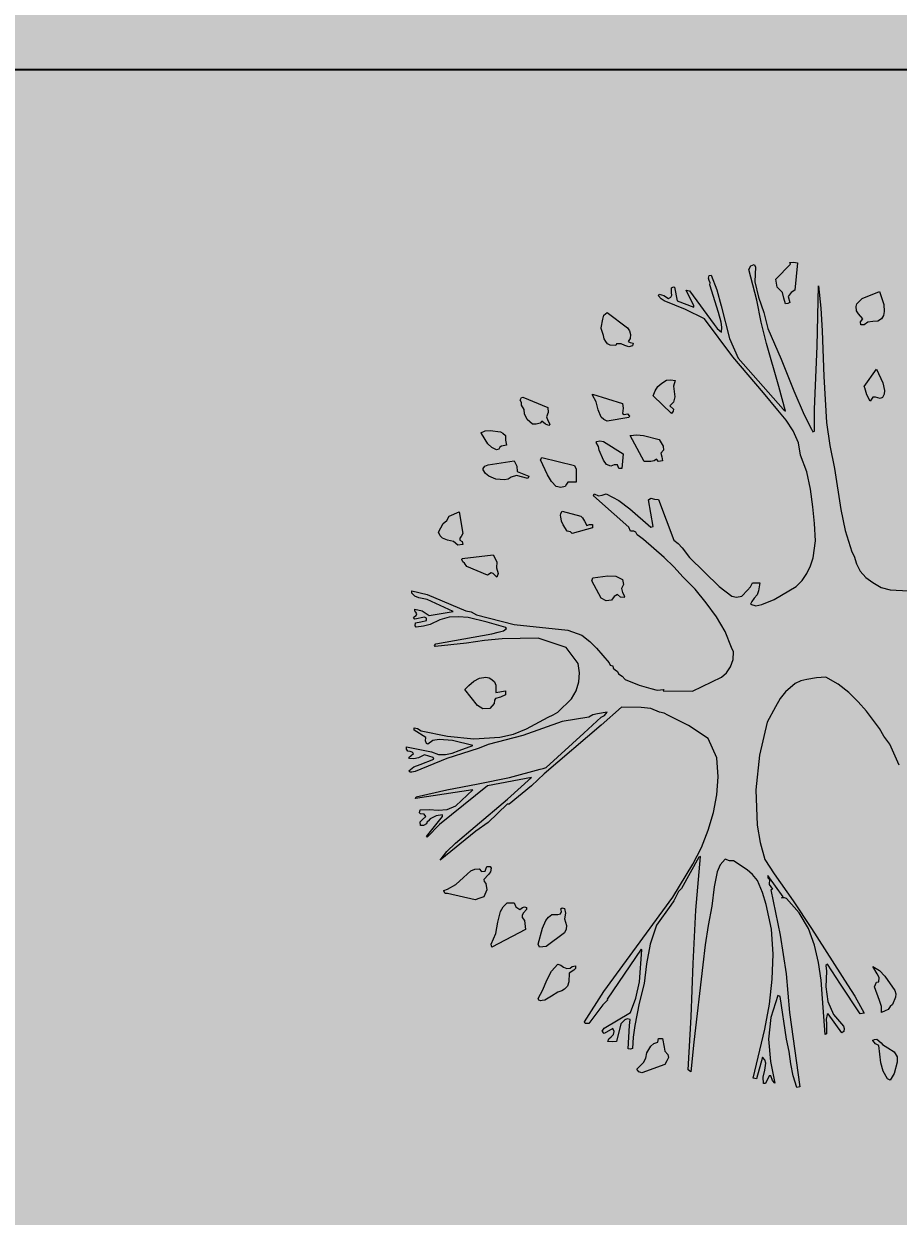
# Model space of a CAD drawing. Units: inches. Extents: x 84 to 1044, y -280 to 906.
# Tile 95 of 105: x 779 to 804, y 479 to 512. Entities that reach past the tile are written whole.
import ezdxf

# ---------------------------------------------------------------- set-up
doc = ezdxf.new("R2010")
doc.units = ezdxf.units.IN
for name, color, linetype, lineweight in [('A-ANNO-DIMS', 2, 'Continuous', 18), ('L-PLNT', 114, 'Continuous', 15), ('WALL', 250, 'Continuous', 35)]:
    doc.layers.add(name, color=color, linetype=linetype, lineweight=lineweight)
doc.layers.add('A-WALL-PATT', color=251, linetype='Continuous', lineweight=9, true_color=0x636466)
doc.layers.add('L-PLNT-PATT', color=9, linetype='Continuous', lineweight=9, true_color=0xafd9aa)
doc.styles.get("Standard").update_dxf_attribs({"font": 'arial.ttf'})
doc.dimstyles.get("Standard").update_dxf_attribs({"dimtxt": 0.18, "dimasz": 0.18, "dimexe": 0.18, "dimexo": 0.0625, "dimgap": 0.09, "dimtad": 0, "dimtih": 1, "dimtoh": 1, "dimdec": 4, "dimzin": 0, "dimdsep": 46, "dimtxsty": 'Standard', "dimcen": 0.09, "dimadec": 0, "dimazin": 0, "dimtfac": 1, "dimtdec": 4, "dimtofl": 0, "dimtmove": 0, "dimatfit": 3, "dimfxl": 1, "dimtolj": 1, "dimtzin": 0, "dimarcsym": 0})

# ---------------------------------------------------------------- blocks, each defined once
blk = doc.blocks.new('A$C37E508DF')
for p, q in [((0.6367, 1.5175), (0.6423, 1.5201)), ((0.6423, 1.5201), (0.6453, 1.5158)), ((0.6826, 1.493), (0.7096, 1.5209)), ((0.7083, 1.5239), (0.7152, 1.5244)), ((0.7096, 1.5209), (0.7083, 1.5239)), ((0.7152, 1.5244), (0.7225, 1.5231)), ((0.7225, 1.5231), (0.7174, 1.4729)), ((0.5583, 1.4948), (0.5596, 1.4995)), ((0.5596, 1.4995), (0.563, 1.5003)), ((0.563, 1.5003), (0.5737, 1.4733)), ((0.6329, 1.5111), (0.6367, 1.5175)), ((0.6475, 1.4545), (0.6329, 1.5111)), ((0.6453, 1.5158), (0.644, 1.4879)), ((0.4897, 1.4772), (0.4935, 1.4789)), ((0.4897, 1.4678), (0.4897, 1.4772)), ((0.4935, 1.4789), (0.4952, 1.478)), ((0.4952, 1.478), (0.5004, 1.4532)), ((0.5596, 1.4905), (0.5583, 1.4948)), ((0.5613, 1.4862), (0.5596, 1.4905)), ((0.5608, 1.4823), (0.5613, 1.4862)), ((0.5767, 1.4317), (0.5608, 1.4823)), ((0.644, 1.4879), (0.6505, 1.46)), ((0.6852, 1.4785), (0.6826, 1.493)), ((0.6946, 1.4682), (0.6852, 1.4785)), ((0.7589, 1.3691), (0.7615, 1.481)), ((0.7615, 1.481), (0.7658, 1.4395)), ((0.4657, 1.4622), (0.4669, 1.4652)), ((0.4708, 1.4566), (0.4657, 1.4622)), ((0.4669, 1.4652), (0.4755, 1.463)), ((0.4764, 1.4532), (0.4708, 1.4566)), ((0.4755, 1.463), (0.4845, 1.4575)), ((0.4845, 1.4575), (0.4884, 1.4596)), ((0.4884, 1.4596), (0.4905, 1.4635)), ((0.4905, 1.4635), (0.4897, 1.4678)), ((0.5313, 1.4437), (0.5167, 1.4729)), ((0.5167, 1.4729), (0.5231, 1.4716)), ((0.5231, 1.4716), (0.5686, 1.409)), ((0.5737, 1.4733), (0.5814, 1.4437)), ((0.6552, 1.4137), (0.6475, 1.4545)), ((0.6505, 1.46), (0.6603, 1.4317)), ((0.6976, 1.4579), (0.6946, 1.4682)), ((0.7002, 1.4476), (0.6976, 1.4579)), ((0.7109, 1.4682), (0.7053, 1.4609)), ((0.7053, 1.4609), (0.7083, 1.4502)), ((0.7174, 1.4729), (0.7109, 1.4682)), ((0.8357, 1.451), (0.8421, 1.4575)), ((0.8421, 1.4575), (0.8739, 1.4703)), ((0.8739, 1.4703), (0.882, 1.4463)), ((0.3649, 1.4266), (0.3709, 1.4317)), ((0.3709, 1.4317), (0.4086, 1.403)), ((0.5154, 1.4373), (0.4764, 1.4532)), ((0.5004, 1.4532), (0.5308, 1.4412)), ((0.551, 1.4197), (0.5154, 1.4373)), ((0.5308, 1.4412), (0.5313, 1.4437)), ((0.5814, 1.4133), (0.5767, 1.4317)), ((0.5814, 1.4437), (0.5969, 1.3833)), ((0.6603, 1.4317), (0.668, 1.4021)), ((0.7049, 1.448), (0.7002, 1.4476)), ((0.7083, 1.4502), (0.7049, 1.448)), ((0.7658, 1.4395), (0.7684, 1.3979)), ((0.831, 1.4424), (0.8323, 1.4476)), ((0.8318, 1.4343), (0.831, 1.4424)), ((0.8353, 1.4292), (0.8318, 1.4343)), ((0.8323, 1.4476), (0.8357, 1.451)), ((0.8829, 1.433), (0.8816, 1.4262)), ((0.882, 1.4463), (0.8829, 1.433)), ((0.3598, 1.403), (0.3628, 1.4189)), ((0.3628, 1.4189), (0.3649, 1.4266)), ((0.6029, 1.3494), (0.551, 1.4197)), ((0.5827, 1.4043), (0.5814, 1.4133)), ((0.6655, 1.3743), (0.6552, 1.4137)), ((0.8434, 1.4197), (0.8353, 1.4292)), ((0.8391, 1.4141), (0.8434, 1.4197)), ((0.8395, 1.4086), (0.8391, 1.4141)), ((0.8528, 1.4137), (0.846, 1.4086)), ((0.8619, 1.4146), (0.8528, 1.4137)), ((0.8709, 1.4154), (0.8619, 1.4146)), ((0.8781, 1.4197), (0.8709, 1.4154)), ((0.8816, 1.4262), (0.8781, 1.4197)), ((0.3602, 1.4021), (0.3598, 1.403)), ((0.364, 1.3888), (0.3602, 1.4021)), ((0.3657, 1.3828), (0.364, 1.3888)), ((0.4086, 1.403), (0.4125, 1.3979)), ((0.4125, 1.3979), (0.4142, 1.391)), ((0.4142, 1.391), (0.4134, 1.3837)), ((0.5686, 1.409), (0.5741, 1.4021)), ((0.5741, 1.4021), (0.5823, 1.3953)), ((0.5823, 1.3953), (0.5827, 1.4043)), ((0.668, 1.4021), (0.6925, 1.3455)), ((0.7684, 1.3979), (0.771, 1.3134)), ((0.846, 1.4086), (0.8395, 1.4086)), ((0.3683, 1.3781), (0.3657, 1.3828)), ((0.3718, 1.3738), (0.3683, 1.3781)), ((0.3765, 1.3713), (0.3718, 1.3738)), ((0.3872, 1.3708), (0.3765, 1.3713)), ((0.3885, 1.3738), (0.3872, 1.3708)), ((0.3971, 1.3734), (0.3885, 1.3738)), ((0.4039, 1.3704), (0.3971, 1.3734)), ((0.4108, 1.3683), (0.4039, 1.3704)), ((0.4134, 1.3837), (0.4099, 1.3781)), ((0.4099, 1.3781), (0.4134, 1.376)), ((0.4176, 1.37), (0.4108, 1.3683)), ((0.4134, 1.376), (0.4189, 1.3751)), ((0.4189, 1.3751), (0.4176, 1.37)), ((0.5969, 1.3833), (0.6132, 1.3472)), ((0.6882, 1.2949), (0.6655, 1.3743)), ((0.7538, 1.2529), (0.7589, 1.3691)), ((0.6595, 1.2829), (0.6029, 1.3494)), ((0.6132, 1.3472), (0.6959, 1.2529)), ((0.6925, 1.3455), (0.7161, 1.2868)), ((0.846, 1.2949), (0.8687, 1.3271)), ((0.8687, 1.3271), (0.8803, 1.3014)), ((0.4648, 1.2945), (0.4717, 1.3009)), ((0.4717, 1.3009), (0.4807, 1.3065)), ((0.4807, 1.3065), (0.4884, 1.3074)), ((0.4884, 1.3074), (0.4965, 1.3057)), ((0.4965, 1.3057), (0.4935, 1.2954)), ((0.771, 1.3134), (0.7761, 1.2285)), ((0.8803, 1.3014), (0.8833, 1.2872)), ((0.3439, 1.2804), (0.3992, 1.2636)), ((0.3439, 1.2787), (0.3439, 1.2804)), ((0.3507, 1.2662), (0.3439, 1.2787)), ((0.4562, 1.2774), (0.4597, 1.2868)), ((0.4897, 1.2452), (0.4562, 1.2774)), ((0.4597, 1.2868), (0.4648, 1.2945)), ((0.4935, 1.2954), (0.4948, 1.2855)), ((0.4948, 1.2855), (0.4961, 1.2756)), ((0.6865, 1.2508), (0.6595, 1.2829)), ((0.7002, 1.2495), (0.6882, 1.2949)), ((0.7161, 1.2868), (0.7349, 1.2422)), ((0.8473, 1.2924), (0.846, 1.2949)), ((0.8507, 1.2795), (0.8473, 1.2924)), ((0.8567, 1.2679), (0.8507, 1.2795)), ((0.8829, 1.2808), (0.8799, 1.2744)), ((0.8833, 1.2872), (0.8829, 1.2808)), ((0.2101, 1.2696), (0.2127, 1.2744)), ((0.2127, 1.2654), (0.2101, 1.2696)), ((0.2127, 1.2744), (0.2152, 1.2752)), ((0.2127, 1.2602), (0.2127, 1.2654)), ((0.2174, 1.2521), (0.2127, 1.2602)), ((0.2152, 1.2752), (0.2611, 1.2559)), ((0.2611, 1.2559), (0.262, 1.2465)), ((0.3546, 1.2516), (0.3507, 1.2662)), ((0.3992, 1.2636), (0.4005, 1.2546)), ((0.4935, 1.2658), (0.4867, 1.2589)), ((0.4867, 1.2589), (0.4935, 1.2529)), ((0.4961, 1.2756), (0.4935, 1.2658)), ((0.8619, 1.2752), (0.8567, 1.2679)), ((0.867, 1.2752), (0.8619, 1.2752)), ((0.8713, 1.2739), (0.867, 1.2752)), ((0.8756, 1.2726), (0.8713, 1.2739)), ((0.8799, 1.2744), (0.8756, 1.2726)), ((0.2182, 1.2443), (0.2174, 1.2521)), ((0.2234, 1.2336), (0.2182, 1.2443)), ((0.2328, 1.2251), (0.2234, 1.2336)), ((0.262, 1.2465), (0.2586, 1.2388)), ((0.2586, 1.2388), (0.2611, 1.2319)), ((0.3602, 1.2383), (0.3546, 1.2516)), ((0.3649, 1.2336), (0.3602, 1.2383)), ((0.3709, 1.2306), (0.3649, 1.2336)), ((0.4112, 1.2375), (0.3709, 1.2306)), ((0.4005, 1.2546), (0.3992, 1.2452)), ((0.3992, 1.2452), (0.4026, 1.2431)), ((0.4026, 1.2431), (0.4086, 1.2443)), ((0.4086, 1.2443), (0.4121, 1.2401)), ((0.4121, 1.2401), (0.4112, 1.2375)), ((0.4931, 1.2491), (0.4897, 1.2452)), ((0.4935, 1.2529), (0.4931, 1.2491)), ((0.7015, 1.2323), (0.6865, 1.2508)), ((0.6959, 1.2529), (0.7002, 1.2495)), ((0.7349, 1.2422), (0.7482, 1.216)), ((0.7538, 1.2122), (0.7538, 1.2529)), ((0.1376, 1.2092), (0.1458, 1.2126)), ((0.1458, 1.2126), (0.1548, 1.2135)), ((0.1548, 1.2135), (0.1741, 1.2109)), ((0.2401, 1.2251), (0.2328, 1.2251)), ((0.2474, 1.2268), (0.2401, 1.2251)), ((0.2504, 1.2306), (0.2474, 1.2268)), ((0.2568, 1.2255), (0.2504, 1.2306)), ((0.2633, 1.2229), (0.2568, 1.2255)), ((0.2611, 1.2319), (0.265, 1.2251)), ((0.265, 1.2251), (0.2633, 1.2229)), ((0.7148, 1.2126), (0.7015, 1.2323)), ((0.7246, 1.1908), (0.7148, 1.2126)), ((0.7482, 1.216), (0.7508, 1.2109)), ((0.7508, 1.2109), (0.7538, 1.2122)), ((0.7761, 1.2285), (0.7821, 1.1856)), ((0.1389, 1.2079), (0.1376, 1.2092)), ((0.1505, 1.189), (0.1389, 1.2079)), ((0.1741, 1.2109), (0.1784, 1.2083)), ((0.1784, 1.2083), (0.1831, 1.204)), ((0.1831, 1.204), (0.1831, 1.1959)), ((0.1831, 1.1959), (0.1848, 1.1865)), ((0.3507, 1.1916), (0.352, 1.1933)), ((0.355, 1.1839), (0.3507, 1.1916)), ((0.352, 1.1933), (0.3576, 1.1942)), ((0.3576, 1.1942), (0.364, 1.1929)), ((0.364, 1.1929), (0.4005, 1.1702)), ((0.4134, 1.204), (0.4258, 1.2058)), ((0.4391, 1.156), (0.4134, 1.204)), ((0.4258, 1.2058), (0.4382, 1.2045)), ((0.4382, 1.2045), (0.4669, 1.1972)), ((0.4669, 1.1972), (0.4747, 1.1843)), ((0.7281, 1.168), (0.7246, 1.1908)), ((0.1582, 1.1822), (0.1505, 1.189)), ((0.1668, 1.1775), (0.1582, 1.1822)), ((0.1711, 1.1792), (0.1668, 1.1775)), ((0.1728, 1.1826), (0.1711, 1.1792)), ((0.1758, 1.1847), (0.1728, 1.1826)), ((0.1788, 1.1852), (0.1758, 1.1847)), ((0.1848, 1.1865), (0.1788, 1.1852)), ((0.3563, 1.177), (0.355, 1.1839)), ((0.3645, 1.1586), (0.3563, 1.177)), ((0.4005, 1.1702), (0.3979, 1.1436)), ((0.4751, 1.177), (0.47, 1.1714)), ((0.47, 1.1714), (0.4721, 1.1646)), ((0.4747, 1.1843), (0.4751, 1.177)), ((0.7396, 1.1371), (0.7281, 1.168)), ((0.7821, 1.1856), (0.7911, 1.1436)), ((0.1419, 1.1436), (0.1449, 1.1474)), ((0.1449, 1.1474), (0.1509, 1.1504)), ((0.1509, 1.1504), (0.1994, 1.1573)), ((0.1994, 1.1573), (0.2041, 1.1479)), ((0.2041, 1.1479), (0.2045, 1.138)), ((0.2478, 1.1594), (0.2504, 1.1637)), ((0.2607, 1.1316), (0.2478, 1.1594)), ((0.2504, 1.1637), (0.3104, 1.1487)), ((0.3104, 1.1487), (0.3134, 1.1423)), ((0.37, 1.1509), (0.3645, 1.1586)), ((0.3778, 1.1474), (0.37, 1.1509)), ((0.3842, 1.15), (0.3778, 1.1474)), ((0.3898, 1.15), (0.3842, 1.15)), ((0.3923, 1.1436), (0.3898, 1.15)), ((0.4519, 1.1564), (0.4391, 1.156)), ((0.458, 1.1573), (0.4519, 1.1564)), ((0.4622, 1.1607), (0.458, 1.1573)), ((0.4657, 1.156), (0.4622, 1.1607)), ((0.473, 1.1573), (0.4657, 1.156)), ((0.4721, 1.1646), (0.473, 1.1573)), ((0.1419, 1.141), (0.1419, 1.1436)), ((0.1462, 1.1342), (0.1419, 1.141)), ((0.1522, 1.1294), (0.1462, 1.1342)), ((0.1655, 1.1234), (0.1522, 1.1294)), ((0.181, 1.1226), (0.1655, 1.1234)), ((0.1878, 1.1234), (0.181, 1.1226)), ((0.1938, 1.1273), (0.1878, 1.1234)), ((0.2032, 1.1303), (0.1938, 1.1273)), ((0.2247, 1.1251), (0.2032, 1.1303)), ((0.2045, 1.138), (0.226, 1.129)), ((0.226, 1.129), (0.2247, 1.1251)), ((0.268, 1.1196), (0.2607, 1.1316)), ((0.3134, 1.1423), (0.3139, 1.1346)), ((0.3139, 1.1346), (0.3134, 1.1183)), ((0.3979, 1.1436), (0.3923, 1.1436)), ((0.7469, 1.1054), (0.7396, 1.1371)), ((0.7911, 1.1436), (0.8027, 1.0677)), ((0.277, 1.1101), (0.268, 1.1196)), ((0.2856, 1.108), (0.277, 1.1101)), ((0.2933, 1.1101), (0.2856, 1.108)), ((0.2959, 1.1144), (0.2933, 1.1101)), ((0.2984, 1.1179), (0.2959, 1.1144)), ((0.3066, 1.1179), (0.2984, 1.1179)), ((0.3134, 1.1183), (0.3066, 1.1179)), ((0.7512, 1.0728), (0.7469, 1.1054)), ((0.3456, 1.093), (0.3469, 1.0964)), ((0.3842, 1.0591), (0.3456, 1.093)), ((0.3469, 1.0964), (0.355, 1.093)), ((0.355, 1.093), (0.3619, 1.0943)), ((0.3619, 1.0943), (0.3692, 1.0968)), ((0.3692, 1.0968), (0.3923, 1.0844)), ((0.3923, 1.0844), (0.4129, 1.069)), ((0.4472, 1.0857), (0.4515, 1.0887)), ((0.4562, 1.0364), (0.4472, 1.0857)), ((0.4515, 1.0887), (0.4584, 1.0865)), ((0.4584, 1.0865), (0.4657, 1.0861)), ((0.4657, 1.0861), (0.4939, 1.0107)), ((0.0789, 1.0552), (0.0978, 1.063)), ((0.0978, 1.063), (0.1042, 1.0231)), ((0.2847, 1.0565), (0.2856, 1.0604)), ((0.2856, 1.0604), (0.2877, 1.0647)), ((0.2877, 1.0647), (0.3224, 1.0552)), ((0.4112, 1.0351), (0.3842, 1.0591)), ((0.4129, 1.069), (0.4515, 1.0351)), ((0.7538, 1.0415), (0.7512, 1.0728)), ((0.8027, 1.0677), (0.8108, 1.0287)), ((0.0596, 1.0257), (0.0682, 1.0415)), ((0.0682, 1.0415), (0.0746, 1.0475)), ((0.0746, 1.0475), (0.0789, 1.0552)), ((0.2851, 1.054), (0.2847, 1.0565)), ((0.2864, 1.0463), (0.2851, 1.054)), ((0.2899, 1.039), (0.2864, 1.0463)), ((0.2972, 1.0274), (0.2899, 1.039)), ((0.3224, 1.0552), (0.3255, 1.0522)), ((0.3255, 1.0522), (0.3293, 1.0458)), ((0.3293, 1.0458), (0.3336, 1.0381)), ((0.3336, 1.0381), (0.3383, 1.0398)), ((0.3383, 1.0398), (0.3439, 1.0402)), ((0.3439, 1.0402), (0.3439, 1.0338)), ((0.4138, 1.0274), (0.4112, 1.0351)), ((0.4515, 1.0351), (0.4562, 1.0364)), ((0.7559, 1.0098), (0.7538, 1.0415)), ((0.0626, 1.0188), (0.0596, 1.0257)), ((0.0665, 1.0149), (0.0626, 1.0188)), ((0.0763, 1.0111), (0.0665, 1.0149)), ((0.1012, 1.018), (0.099, 1.0149)), ((0.099, 1.0149), (0.099, 1.0111)), ((0.1042, 1.0231), (0.1012, 1.018)), ((0.3032, 1.0265), (0.2972, 1.0274)), ((0.3066, 1.0231), (0.3032, 1.0265)), ((0.3439, 1.0338), (0.3066, 1.0231)), ((0.4202, 1.0274), (0.4138, 1.0274)), ((0.4241, 1.0257), (0.4202, 1.0274)), ((0.4267, 1.0209), (0.4241, 1.0257)), ((0.4305, 1.0175), (0.4267, 1.0209)), ((0.4378, 1.0124), (0.4305, 1.0175)), ((0.8108, 1.0287), (0.8233, 0.9892)), ((0.087, 1.0085), (0.0763, 1.0111)), ((0.0948, 1.0016), (0.087, 1.0085)), ((0.1042, 1.0029), (0.0948, 1.0016)), ((0.099, 1.0111), (0.1033, 1.0085)), ((0.1033, 1.0085), (0.1042, 1.0029)), ((0.476, 0.9789), (0.4378, 1.0124)), ((0.4939, 1.0107), (0.5021, 1.0051)), ((0.5021, 1.0051), (0.5094, 0.9969)), ((0.5094, 0.9969), (0.5231, 0.9789)), ((0.7516, 0.9785), (0.7559, 1.0098)), ((0.1025, 0.9751), (0.1029, 0.9772)), ((0.1046, 0.9708), (0.1025, 0.9751)), ((0.1029, 0.9772), (0.1604, 0.9841)), ((0.1076, 0.9682), (0.1046, 0.9708)), ((0.1604, 0.9841), (0.1672, 0.9708)), ((0.1672, 0.9708), (0.1664, 0.9601)), ((0.4939, 0.9618), (0.476, 0.9789)), ((0.5231, 0.9789), (0.578, 0.9253)), ((0.7469, 0.9635), (0.7516, 0.9785)), ((0.8233, 0.9892), (0.8275, 0.9815)), ((0.8275, 0.9815), (0.8314, 0.9673)), ((0.1119, 0.9626), (0.1076, 0.9682)), ((0.1496, 0.9463), (0.1119, 0.9626)), ((0.1565, 0.9506), (0.1496, 0.9463)), ((0.1604, 0.9493), (0.1565, 0.9506)), ((0.1629, 0.9468), (0.1604, 0.9493)), ((0.1664, 0.9601), (0.1698, 0.9493)), ((0.1698, 0.9493), (0.1672, 0.9429)), ((0.5111, 0.9429), (0.4939, 0.9618)), ((0.7315, 0.9365), (0.7401, 0.9493)), ((0.7401, 0.9493), (0.7469, 0.9635)), ((0.8314, 0.9673), (0.8383, 0.954)), ((0.8383, 0.954), (0.8486, 0.942)), ((0.1672, 0.9429), (0.1629, 0.9468)), ((0.3426, 0.936), (0.3443, 0.9412)), ((0.3602, 0.9039), (0.3426, 0.936)), ((0.3443, 0.9412), (0.3722, 0.9451)), ((0.3722, 0.9451), (0.3868, 0.9446)), ((0.3868, 0.9446), (0.3992, 0.9386)), ((0.4009, 0.9292), (0.3975, 0.9215)), ((0.3992, 0.9386), (0.4009, 0.9292)), ((0.5334, 0.9202), (0.5111, 0.9429)), ((0.578, 0.9253), (0.6011, 0.9077)), ((0.6359, 0.9245), (0.6397, 0.9322)), ((0.6397, 0.9322), (0.653, 0.9322)), ((0.653, 0.9322), (0.6505, 0.9172)), ((0.6796, 0.9013), (0.7203, 0.9253)), ((0.7203, 0.9253), (0.7315, 0.9365)), ((0.8486, 0.942), (0.8619, 0.933)), ((0.8619, 0.933), (0.8769, 0.9236)), ((0.0103, 0.9129), (0.0103, 0.9172)), ((0.0103, 0.9172), (0.0382, 0.9107)), ((0.0159, 0.9073), (0.0103, 0.9129)), ((0.0232, 0.9043), (0.0159, 0.9073)), ((0.0386, 0.9013), (0.0232, 0.9043)), ((0.0382, 0.9107), (0.1098, 0.8807)), ((0.3692, 0.8992), (0.3602, 0.9039)), ((0.3838, 0.9069), (0.379, 0.9)), ((0.3898, 0.9107), (0.3838, 0.9069)), ((0.3958, 0.906), (0.3898, 0.9107)), ((0.4026, 0.9052), (0.3958, 0.906)), ((0.3975, 0.9215), (0.3996, 0.9142)), ((0.3996, 0.9142), (0.4031, 0.9077)), ((0.4031, 0.9077), (0.4026, 0.9052)), ((0.554, 0.8953), (0.5334, 0.9202)), ((0.6011, 0.9077), (0.6097, 0.9056)), ((0.6097, 0.9056), (0.6196, 0.9077)), ((0.6196, 0.9077), (0.6303, 0.9189)), ((0.6303, 0.9189), (0.6359, 0.9245)), ((0.6423, 0.9039), (0.6384, 0.8974)), ((0.6479, 0.9103), (0.6423, 0.9039)), ((0.6505, 0.9172), (0.6479, 0.9103)), ((0.8769, 0.9236), (0.8936, 0.9193)), ((0.8936, 0.9193), (0.9279, 0.9172)), ((0.0159, 0.8803), (0.0154, 0.8837)), ((0.0154, 0.8837), (0.0292, 0.8803)), ((0.0866, 0.8794), (0.0386, 0.9013)), ((0.379, 0.9), (0.3692, 0.8992)), ((0.5728, 0.8691), (0.554, 0.8953)), ((0.6384, 0.8974), (0.6359, 0.8927)), ((0.6359, 0.8927), (0.6457, 0.8897)), ((0.6457, 0.8897), (0.6569, 0.8919)), ((0.6569, 0.8919), (0.6796, 0.9013)), ((0.0133, 0.8679), (0.015, 0.87)), ((0.0154, 0.8649), (0.0133, 0.8679)), ((0.015, 0.87), (0.0184, 0.8717)), ((0.0334, 0.8687), (0.0154, 0.8649)), ((0.0176, 0.8777), (0.0159, 0.8803)), ((0.0171, 0.8584), (0.0266, 0.8602)), ((0.0193, 0.8752), (0.0176, 0.8777)), ((0.0184, 0.8717), (0.0193, 0.8752)), ((0.0266, 0.8602), (0.0369, 0.8623)), ((0.0292, 0.8803), (0.0424, 0.8717)), ((0.0369, 0.8666), (0.0334, 0.8687)), ((0.0369, 0.8623), (0.0369, 0.8666)), ((0.0424, 0.8717), (0.0866, 0.8794)), ((0.0617, 0.864), (0.0442, 0.8554)), ((0.0789, 0.8687), (0.0617, 0.864)), ((0.0965, 0.8696), (0.0789, 0.8687)), ((0.1141, 0.8679), (0.0965, 0.8696)), ((0.1098, 0.8807), (0.1196, 0.8786)), ((0.1492, 0.8593), (0.1141, 0.8679)), ((0.1196, 0.8786), (0.1295, 0.873)), ((0.1295, 0.873), (0.1994, 0.8554)), ((0.1835, 0.8499), (0.1492, 0.8593)), ((0.5887, 0.8421), (0.5728, 0.8691)), ((0.0163, 0.8529), (0.0171, 0.8584)), ((0.0184, 0.8503), (0.0163, 0.8529)), ((0.0317, 0.8524), (0.0184, 0.8503)), ((0.0442, 0.8554), (0.0317, 0.8524)), ((0.0545, 0.8194), (0.1578, 0.8378)), ((0.1578, 0.8378), (0.1698, 0.8413)), ((0.1698, 0.8413), (0.1792, 0.8434)), ((0.1792, 0.8434), (0.1848, 0.8477)), ((0.1848, 0.8477), (0.1835, 0.8499)), ((0.1994, 0.8554), (0.2984, 0.8447)), ((0.2984, 0.8447), (0.3242, 0.8357)), ((0.6007, 0.8125), (0.5887, 0.8421)), ((0.0519, 0.8164), (0.0545, 0.8194)), ((0.0532, 0.8143), (0.0519, 0.8164)), ((0.1111, 0.8207), (0.0532, 0.8143)), ((0.1441, 0.8258), (0.1111, 0.8207)), ((0.1771, 0.8288), (0.1441, 0.8258)), ((0.2436, 0.8301), (0.1771, 0.8288)), ((0.2954, 0.813), (0.2436, 0.8301)), ((0.3242, 0.8357), (0.3387, 0.8241)), ((0.3387, 0.8241), (0.3512, 0.8117)), ((0.3173, 0.7834), (0.2954, 0.813)), ((0.3512, 0.8117), (0.3748, 0.7842)), ((0.6046, 0.8048), (0.6007, 0.8125)), ((0.6037, 0.7903), (0.6046, 0.8048)), ((0.3199, 0.7662), (0.3173, 0.7834)), ((0.3748, 0.7842), (0.3765, 0.7804)), ((0.3765, 0.7804), (0.3816, 0.7791)), ((0.3816, 0.7791), (0.382, 0.7744)), ((0.382, 0.7744), (0.3859, 0.7714)), ((0.3859, 0.7714), (0.3902, 0.7684)), ((0.5913, 0.7658), (0.599, 0.777)), ((0.599, 0.777), (0.6037, 0.7903)), ((0.1153, 0.7427), (0.1244, 0.7504)), ((0.1244, 0.7504), (0.1351, 0.7559)), ((0.1351, 0.7559), (0.1471, 0.7577)), ((0.1471, 0.7577), (0.1527, 0.7568)), ((0.1527, 0.7568), (0.1578, 0.7538)), ((0.1578, 0.7538), (0.1629, 0.7491)), ((0.1629, 0.7491), (0.1651, 0.7431)), ((0.3139, 0.7324), (0.3186, 0.7491)), ((0.3186, 0.7491), (0.3199, 0.7662)), ((0.3902, 0.7684), (0.3919, 0.7641)), ((0.3919, 0.7641), (0.3988, 0.7598)), ((0.3988, 0.7598), (0.4043, 0.7538)), ((0.4043, 0.7538), (0.4301, 0.7431)), ((0.5287, 0.7319), (0.5823, 0.7577)), ((0.5823, 0.7577), (0.5913, 0.7658)), ((0.7285, 0.7512), (0.7182, 0.7461)), ((0.7401, 0.7534), (0.7285, 0.7512)), ((0.7577, 0.7568), (0.7401, 0.7534)), ((0.7752, 0.7577), (0.7577, 0.7568)), ((0.798, 0.7452), (0.7752, 0.7577)), ((0.1081, 0.7349), (0.1153, 0.7427)), ((0.1312, 0.7058), (0.1081, 0.7349)), ((0.1651, 0.7431), (0.1655, 0.7298)), ((0.1655, 0.7298), (0.1831, 0.7324)), ((0.1831, 0.7324), (0.1831, 0.7255)), ((0.3049, 0.7178), (0.3139, 0.7324)), ((0.4301, 0.7431), (0.4515, 0.7371)), ((0.4515, 0.7371), (0.4635, 0.7341)), ((0.4635, 0.7341), (0.4755, 0.7349)), ((0.4755, 0.7349), (0.4742, 0.7324)), ((0.4742, 0.7324), (0.5287, 0.7319)), ((0.7002, 0.7307), (0.6903, 0.7186)), ((0.7182, 0.7461), (0.7002, 0.7307)), ((0.8173, 0.7298), (0.798, 0.7452)), ((0.8344, 0.7122), (0.8173, 0.7298)), ((0.1415, 0.6994), (0.1312, 0.7058)), ((0.1621, 0.7092), (0.1539, 0.7002)), ((0.1629, 0.7152), (0.1621, 0.7092)), ((0.1646, 0.7186), (0.1629, 0.7152)), ((0.1741, 0.7208), (0.1646, 0.7186)), ((0.1831, 0.7255), (0.1741, 0.7208)), ((0.28, 0.6933), (0.3049, 0.7178)), ((0.6903, 0.7186), (0.6818, 0.7032)), ((0.8503, 0.6951), (0.8344, 0.7122)), ((0.1539, 0.7002), (0.1415, 0.6994)), ((0.2221, 0.6625), (0.262, 0.6839)), ((0.262, 0.6839), (0.271, 0.6882)), ((0.271, 0.6882), (0.28, 0.6933)), ((0.337, 0.6843), (0.2877, 0.6762)), ((0.328, 0.6543), (0.3598, 0.6843)), ((0.3443, 0.6886), (0.337, 0.6843)), ((0.3533, 0.6903), (0.3443, 0.6886)), ((0.3709, 0.6933), (0.3533, 0.6903)), ((0.3975, 0.7028), (0.3598, 0.6693)), ((0.3598, 0.6843), (0.3662, 0.6873)), ((0.3662, 0.6873), (0.3709, 0.6933)), ((0.4339, 0.7019), (0.3975, 0.7028)), ((0.4515, 0.7002), (0.4339, 0.7019)), ((0.4674, 0.6933), (0.4515, 0.7002)), ((0.476, 0.6912), (0.4674, 0.6933)), ((0.4832, 0.6878), (0.476, 0.6912)), ((0.521, 0.6685), (0.4832, 0.6878)), ((0.6818, 0.7032), (0.6667, 0.6749)), ((0.8739, 0.6629), (0.8503, 0.6951)), ((0.0146, 0.6599), (0.0146, 0.6642)), ((0.0146, 0.6642), (0.0206, 0.6633)), ((0.0206, 0.6633), (0.0274, 0.6586)), ((0.1977, 0.6526), (0.2221, 0.6625)), ((0.2877, 0.6762), (0.2152, 0.6505)), ((0.3598, 0.6693), (0.2543, 0.5797)), ((0.5578, 0.6449), (0.521, 0.6685)), ((0.6667, 0.6749), (0.6526, 0.614)), ((0.8824, 0.6492), (0.8739, 0.6629)), ((0.036, 0.6466), (0.0146, 0.6599)), ((0.0274, 0.6586), (0.0759, 0.6492)), ((0.0356, 0.6406), (0.036, 0.6466)), ((0.0369, 0.6355), (0.0356, 0.6406)), ((0.0489, 0.641), (0.0399, 0.6342)), ((0.0609, 0.6428), (0.0489, 0.641)), ((0.0853, 0.641), (0.0609, 0.6428)), ((0.0759, 0.6492), (0.1244, 0.644)), ((0.1226, 0.632), (0.0853, 0.641)), ((0.1244, 0.644), (0.1728, 0.647)), ((0.2152, 0.6505), (0.1509, 0.6333)), ((0.1728, 0.647), (0.1977, 0.6526)), ((0.2581, 0.5913), (0.328, 0.6543)), ((0.5737, 0.6089), (0.5578, 0.6449)), ((0.8932, 0.6342), (0.8824, 0.6492)), ((0, 0.629), (0.0467, 0.62)), ((0, 0.6252), (0, 0.629)), ((0.003, 0.6213), (0, 0.6252)), ((0.0069, 0.6204), (0.003, 0.6213)), ((0.0107, 0.6196), (0.0069, 0.6204)), ((0.0086, 0.6132), (0.0133, 0.617)), ((0.0133, 0.617), (0.0107, 0.6196)), ((0.0399, 0.6342), (0.0369, 0.6355)), ((0.0467, 0.62), (0.0592, 0.6153)), ((0.072, 0.6149), (0.0849, 0.6175)), ((0.1175, 0.6213), (0.0746, 0.6076)), ((0.0849, 0.6175), (0.0973, 0.6226)), ((0.0973, 0.6226), (0.1226, 0.632)), ((0.1342, 0.6265), (0.1175, 0.6213)), ((0.1509, 0.6333), (0.1342, 0.6265)), ((0.9103, 0.5956), (0.8932, 0.6342)), ((0.0047, 0.6093), (0.0086, 0.6132)), ((0.0056, 0.6076), (0.0047, 0.6093)), ((0.0141, 0.6072), (0.0056, 0.6076)), ((0.0223, 0.6089), (0.0141, 0.6072)), ((0.0141, 0.5921), (0.0257, 0.5969)), ((0.0746, 0.6076), (0.0163, 0.5836)), ((0.0334, 0.6145), (0.0223, 0.6089)), ((0.0257, 0.5969), (0.0506, 0.6063)), ((0.0416, 0.6119), (0.0334, 0.6145)), ((0.0493, 0.6093), (0.0416, 0.6119)), ((0.0506, 0.6063), (0.0493, 0.6093)), ((0.0592, 0.6153), (0.072, 0.6149)), ((0.5763, 0.5741), (0.5737, 0.6089)), ((0.6526, 0.614), (0.6457, 0.5497)), ((0.0047, 0.5849), (0.0141, 0.5921)), ((0.0069, 0.5823), (0.0047, 0.5849)), ((0.0099, 0.5823), (0.0069, 0.5823)), ((0.0163, 0.5836), (0.0099, 0.5823)), ((0.2311, 0.5729), (0.1496, 0.557)), ((0.1869, 0.5325), (0.2311, 0.5729)), ((0.1904, 0.5724), (0.2474, 0.5879)), ((0.2543, 0.5797), (0.2311, 0.557)), ((0.2474, 0.5879), (0.253, 0.5892)), ((0.253, 0.5892), (0.2581, 0.5913)), ((0.5737, 0.5407), (0.5763, 0.5741)), ((0.1496, 0.557), (0.0613, 0.4858)), ((0.0746, 0.5501), (0.1325, 0.5608)), ((0.1325, 0.5608), (0.1904, 0.5724)), ((0.2311, 0.557), (0.1899, 0.5235)), ((0.1226, 0.5497), (0.0171, 0.5338)), ((0.0171, 0.5338), (0.0184, 0.5368)), ((0.0184, 0.5368), (0.0746, 0.5501)), ((0.0917, 0.5205), (0.1226, 0.5497)), ((0.1269, 0.482), (0.1869, 0.5325)), ((0.5677, 0.5077), (0.5737, 0.5407)), ((0.6457, 0.5497), (0.6483, 0.4845)), ((0.024, 0.5072), (0.0253, 0.5128)), ((0.0262, 0.5055), (0.024, 0.5072)), ((0.0253, 0.5128), (0.042, 0.5133)), ((0.042, 0.5133), (0.0587, 0.5124)), ((0.0587, 0.5124), (0.0755, 0.5133)), ((0.0755, 0.5133), (0.0917, 0.5205)), ((0.1861, 0.5231), (0.1509, 0.4897)), ((0.1899, 0.5235), (0.1861, 0.5231)), ((0.5578, 0.4751), (0.5677, 0.5077)), ((0.0253, 0.491), (0.03, 0.4948)), ((0.0262, 0.4841), (0.0253, 0.491)), ((0.0326, 0.5047), (0.0262, 0.5055)), ((0.03, 0.4948), (0.036, 0.5004)), ((0.0369, 0.4871), (0.0317, 0.4841)), ((0.036, 0.5004), (0.0326, 0.5047)), ((0.0369, 0.4639), (0.0669, 0.5004)), ((0.0382, 0.4905), (0.0369, 0.4871)), ((0.0403, 0.4922), (0.0382, 0.4905)), ((0.0613, 0.4858), (0.0386, 0.4627)), ((0.0437, 0.4961), (0.0403, 0.4922)), ((0.0549, 0.5021), (0.0437, 0.4961)), ((0.0669, 0.5034), (0.0549, 0.5021)), ((0.0669, 0.5004), (0.0669, 0.5034)), ((0.1509, 0.4897), (0.1282, 0.4734)), ((0.6483, 0.4845), (0.6539, 0.4524)), ((0.0317, 0.4841), (0.0262, 0.4841)), ((0.0386, 0.4627), (0.0369, 0.4639)), ((0.1282, 0.4734), (0.0626, 0.4198)), ((0.0905, 0.4515), (0.1269, 0.482)), ((0.545, 0.4434), (0.5578, 0.4751)), ((0.0746, 0.4361), (0.0905, 0.4515)), ((0.5295, 0.4125), (0.545, 0.4434)), ((0.6539, 0.4524), (0.6625, 0.4211)), ((0.0626, 0.4198), (0.0746, 0.4361)), ((0.5403, 0.4254), (0.5081, 0.3679)), ((0.5347, 0.3276), (0.5433, 0.4266)), ((0.5433, 0.4266), (0.5403, 0.4254)), ((0.5887, 0.4215), (0.5797, 0.4112)), ((0.5969, 0.4189), (0.5887, 0.4215)), ((0.6046, 0.4189), (0.5969, 0.4189)), ((0.6295, 0.4022), (0.6046, 0.4189)), ((0.6625, 0.4211), (0.6796, 0.3945)), ((0.1055, 0.388), (0.1192, 0.4001)), ((0.1192, 0.4001), (0.1265, 0.4031)), ((0.1265, 0.4031), (0.1346, 0.4039)), ((0.1346, 0.4039), (0.1389, 0.3992)), ((0.1389, 0.3992), (0.1458, 0.3996)), ((0.1458, 0.3996), (0.1471, 0.4035)), ((0.1471, 0.4035), (0.1484, 0.4082)), ((0.1484, 0.4082), (0.1548, 0.4082)), ((0.1556, 0.3983), (0.1518, 0.3932)), ((0.1548, 0.4082), (0.1565, 0.4052)), ((0.1565, 0.4052), (0.1556, 0.3983)), ((0.4922, 0.3516), (0.5295, 0.4125)), ((0.5741, 0.3983), (0.5686, 0.3705)), ((0.5797, 0.4112), (0.5741, 0.3983)), ((0.6397, 0.3936), (0.6295, 0.4022)), ((0.0763, 0.3662), (0.0917, 0.3748)), ((0.0917, 0.3748), (0.1055, 0.388)), ((0.1518, 0.3932), (0.1432, 0.3842)), ((0.1432, 0.3842), (0.1436, 0.3808)), ((0.1436, 0.3808), (0.1471, 0.3769)), ((0.1471, 0.3769), (0.1484, 0.3649)), ((0.6487, 0.3825), (0.6397, 0.3936)), ((0.6582, 0.3602), (0.6487, 0.3825)), ((0.6959, 0.352), (0.668, 0.3919)), ((0.668, 0.3919), (0.668, 0.3872)), ((0.668, 0.3872), (0.6706, 0.3842)), ((0.6706, 0.3842), (0.6702, 0.3748)), ((0.6702, 0.3748), (0.6762, 0.3662)), ((0.6796, 0.3945), (0.7148, 0.3447)), ((0.069, 0.364), (0.0763, 0.3662)), ((0.069, 0.3627), (0.069, 0.364)), ((0.0716, 0.3585), (0.069, 0.3627)), ((0.0763, 0.3585), (0.0716, 0.3585)), ((0.1269, 0.3464), (0.0763, 0.3585)), ((0.1484, 0.3649), (0.1432, 0.352)), ((0.4982, 0.3537), (0.4939, 0.3447)), ((0.5025, 0.3619), (0.4982, 0.3537)), ((0.5081, 0.3679), (0.5025, 0.3619)), ((0.5686, 0.3705), (0.5643, 0.3349)), ((0.665, 0.3379), (0.6582, 0.3602)), ((0.6762, 0.3662), (0.6732, 0.3653)), ((0.6732, 0.3653), (0.6903, 0.2813)), ((0.1355, 0.3499), (0.1269, 0.3464)), ((0.1432, 0.352), (0.1355, 0.3499)), ((0.1737, 0.325), (0.1788, 0.3336)), ((0.1788, 0.3336), (0.1861, 0.3409)), ((0.1861, 0.3409), (0.199, 0.3409)), ((0.199, 0.3409), (0.2024, 0.3336)), ((0.2024, 0.3336), (0.2097, 0.3289)), ((0.2097, 0.3289), (0.2148, 0.3323)), ((0.2148, 0.3323), (0.2182, 0.3336)), ((0.2182, 0.3336), (0.2221, 0.3327)), ((0.2221, 0.3327), (0.2221, 0.3289)), ((0.2851, 0.3302), (0.2877, 0.3319)), ((0.2877, 0.3319), (0.292, 0.3306)), ((0.292, 0.3306), (0.2941, 0.322)), ((0.4065, 0.2345), (0.4922, 0.3516)), ((0.4884, 0.337), (0.4622, 0.2997)), ((0.4939, 0.3447), (0.4884, 0.337)), ((0.5643, 0.3349), (0.5578, 0.2993)), ((0.6745, 0.2924), (0.665, 0.3379)), ((0.6933, 0.3503), (0.6959, 0.352)), ((0.6985, 0.3503), (0.6933, 0.3503)), ((0.7023, 0.349), (0.6985, 0.3503)), ((0.7259, 0.3224), (0.7023, 0.349)), ((0.7148, 0.3447), (0.7487, 0.2937)), ((0.1689, 0.3053), (0.1737, 0.325)), ((0.2161, 0.3224), (0.214, 0.3186)), ((0.214, 0.3186), (0.214, 0.3139)), ((0.214, 0.3139), (0.2182, 0.3087)), ((0.2221, 0.3289), (0.2161, 0.3224)), ((0.2182, 0.3087), (0.2204, 0.292)), ((0.2517, 0.2946), (0.2577, 0.3087)), ((0.2577, 0.3087), (0.2624, 0.3147)), ((0.2624, 0.3147), (0.2689, 0.3194)), ((0.2689, 0.3194), (0.2796, 0.3194)), ((0.2796, 0.3194), (0.2847, 0.3211)), ((0.2847, 0.3211), (0.2864, 0.325)), ((0.2864, 0.325), (0.2851, 0.3302)), ((0.2941, 0.322), (0.292, 0.3117)), ((0.292, 0.3117), (0.2959, 0.2993)), ((0.53, 0.229), (0.5347, 0.3276)), ((0.7427, 0.2937), (0.7259, 0.3224)), ((0.2204, 0.292), (0.1578, 0.259)), ((0.1655, 0.2843), (0.1689, 0.3053)), ((0.2436, 0.265), (0.2517, 0.2946)), ((0.2954, 0.2928), (0.292, 0.286)), ((0.2959, 0.2993), (0.2954, 0.2928)), ((0.4622, 0.2997), (0.4502, 0.2645)), ((0.5578, 0.2993), (0.5518, 0.2633)), ((0.6775, 0.2465), (0.6745, 0.2924)), ((0.7542, 0.2628), (0.7427, 0.2937)), ((0.7487, 0.2937), (0.8151, 0.1899)), ((0.1565, 0.265), (0.1655, 0.2843)), ((0.1578, 0.259), (0.1565, 0.265)), ((0.2461, 0.259), (0.2436, 0.265)), ((0.292, 0.286), (0.2581, 0.2607)), ((0.4502, 0.2645), (0.4438, 0.2285)), ((0.6903, 0.2813), (0.7015, 0.2101)), ((0.2581, 0.2607), (0.2461, 0.259)), ((0.4335, 0.2556), (0.3709, 0.1634)), ((0.4305, 0.1951), (0.4352, 0.2543)), ((0.4352, 0.2543), (0.4335, 0.2556)), ((0.5518, 0.2633), (0.5475, 0.2268)), ((0.6758, 0.2002), (0.6775, 0.2465)), ((0.7615, 0.2311), (0.7542, 0.2628)), ((0.268, 0.2148), (0.28, 0.2277)), ((0.28, 0.2277), (0.2851, 0.226)), ((0.2851, 0.226), (0.2903, 0.2225)), ((0.2903, 0.2225), (0.2963, 0.22)), ((0.2963, 0.22), (0.3027, 0.2204)), ((0.3027, 0.2204), (0.3061, 0.2234)), ((0.3061, 0.2234), (0.3122, 0.2247)), ((0.3122, 0.2247), (0.3122, 0.22)), ((0.3649, 0.1775), (0.4065, 0.2345)), ((0.4438, 0.2285), (0.4391, 0.1921)), ((0.5261, 0.1308), (0.53, 0.229)), ((0.5475, 0.2268), (0.5313, 0.084)), ((0.7662, 0.1981), (0.7615, 0.2311)), ((0.7778, 0.2277), (0.7752, 0.2255)), ((0.7752, 0.2255), (0.7761, 0.2152)), ((0.8018, 0.1912), (0.7778, 0.2277)), ((0.8619, 0.2234), (0.8739, 0.2161)), ((0.87, 0.2101), (0.8619, 0.2234)), ((0.2594, 0.1981), (0.268, 0.2148)), ((0.301, 0.211), (0.3002, 0.1951)), ((0.3096, 0.2165), (0.301, 0.211)), ((0.3122, 0.22), (0.3096, 0.2165)), ((0.6706, 0.1539), (0.6758, 0.2002)), ((0.7015, 0.2101), (0.7079, 0.1389)), ((0.7761, 0.2152), (0.7752, 0.1861)), ((0.8734, 0.2032), (0.87, 0.2101)), ((0.8726, 0.1955), (0.8734, 0.2032)), ((0.8739, 0.2161), (0.8841, 0.2054)), ((0.8841, 0.2054), (0.9026, 0.1792)), ((0.2436, 0.1642), (0.2521, 0.1805)), ((0.2521, 0.1805), (0.2594, 0.1981)), ((0.28, 0.1762), (0.2684, 0.1689)), ((0.2873, 0.1788), (0.28, 0.1762)), ((0.292, 0.1818), (0.2873, 0.1788)), ((0.298, 0.1874), (0.292, 0.1818)), ((0.3002, 0.1951), (0.298, 0.1874)), ((0.3293, 0.1213), (0.3649, 0.1775)), ((0.4241, 0.1651), (0.4305, 0.1951)), ((0.4391, 0.1921), (0.4301, 0.1561)), ((0.7688, 0.1646), (0.7662, 0.1981)), ((0.7752, 0.1861), (0.7787, 0.1591)), ((0.8383, 0.1359), (0.8018, 0.1912)), ((0.8151, 0.1899), (0.8288, 0.1685)), ((0.8649, 0.1857), (0.8687, 0.1947)), ((0.8743, 0.1608), (0.8649, 0.1857)), ((0.8687, 0.1947), (0.8726, 0.1955)), ((0.9026, 0.1792), (0.9043, 0.1732)), ((0.2448, 0.1616), (0.2436, 0.1642)), ((0.2478, 0.1599), (0.2448, 0.1616)), ((0.2508, 0.1608), (0.2478, 0.1599)), ((0.2556, 0.1616), (0.2508, 0.1608)), ((0.2684, 0.1689), (0.2556, 0.1616)), ((0.3692, 0.1591), (0.3628, 0.1526)), ((0.3718, 0.1616), (0.3692, 0.1591)), ((0.3709, 0.1634), (0.3718, 0.1616)), ((0.4138, 0.1389), (0.4241, 0.1651)), ((0.4301, 0.1561), (0.4224, 0.1145)), ((0.6865, 0.1698), (0.6732, 0.1295)), ((0.6903, 0.1681), (0.6865, 0.1698)), ((0.7023, 0.0892), (0.6903, 0.1681)), ((0.774, 0.0982), (0.7688, 0.1646)), ((0.7787, 0.1591), (0.789, 0.1346)), ((0.8288, 0.1685), (0.846, 0.1376)), ((0.8777, 0.1496), (0.8743, 0.1608)), ((0.9035, 0.1668), (0.8983, 0.1535)), ((0.9043, 0.1732), (0.9035, 0.1668)), ((0.3628, 0.1526), (0.337, 0.1183)), ((0.3653, 0.1098), (0.4138, 0.1389)), ((0.662, 0.108), (0.6706, 0.1539)), ((0.7079, 0.1389), (0.7268, 0.0013)), ((0.7774, 0.1346), (0.7757, 0.1261)), ((0.7791, 0.1359), (0.7774, 0.1346)), ((0.8044, 0.1012), (0.7791, 0.1359)), ((0.789, 0.1346), (0.8074, 0.1132)), ((0.846, 0.1376), (0.8383, 0.1359)), ((0.8781, 0.1389), (0.8777, 0.1496)), ((0.8846, 0.1419), (0.8781, 0.1389)), ((0.8902, 0.1441), (0.8846, 0.1419)), ((0.894, 0.1496), (0.8902, 0.1441)), ((0.8983, 0.1535), (0.894, 0.1496)), ((0.3306, 0.1183), (0.3293, 0.1213)), ((0.337, 0.1183), (0.3306, 0.1183)), ((0.3962, 0.1175), (0.3885, 0.0853)), ((0.4039, 0.1248), (0.3962, 0.1175)), ((0.4082, 0.1269), (0.4039, 0.1248)), ((0.4134, 0.1256), (0.4082, 0.1269)), ((0.4099, 0.0716), (0.4121, 0.1145)), ((0.4121, 0.1145), (0.4134, 0.1256)), ((0.4224, 0.1145), (0.4189, 0.093)), ((0.5205, 0.033), (0.5261, 0.1308)), ((0.6732, 0.1295), (0.6693, 0.0892)), ((0.7757, 0.1261), (0.7761, 0.117)), ((0.7761, 0.117), (0.7761, 0.099)), ((0.8074, 0.1132), (0.8087, 0.1089)), ((0.3615, 0.1042), (0.3653, 0.1098)), ((0.3653, 0.0999), (0.3615, 0.1042)), ((0.3812, 0.1089), (0.3653, 0.0999)), ((0.3722, 0.0853), (0.3739, 0.09)), ((0.3739, 0.09), (0.3782, 0.0935)), ((0.3782, 0.0935), (0.3825, 0.0978)), ((0.3842, 0.1037), (0.3812, 0.1089)), ((0.3825, 0.0978), (0.3842, 0.1037)), ((0.4189, 0.093), (0.4176, 0.072)), ((0.4648, 0.084), (0.4657, 0.0905)), ((0.4657, 0.0905), (0.473, 0.0905)), ((0.473, 0.0905), (0.476, 0.0746)), ((0.641, 0.0172), (0.662, 0.108)), ((0.6693, 0.0892), (0.6728, 0.0484)), ((0.7075, 0.0665), (0.7023, 0.0892)), ((0.7761, 0.099), (0.774, 0.0982)), ((0.8083, 0.1037), (0.8044, 0.1012)), ((0.8087, 0.1089), (0.8083, 0.1037)), ((0.8619, 0.0875), (0.8649, 0.0887)), ((0.8649, 0.0887), (0.8691, 0.0892)), ((0.8691, 0.0892), (0.8769, 0.0827)), ((0.3808, 0.0845), (0.3722, 0.0853)), ((0.3885, 0.0853), (0.3808, 0.0845)), ((0.4142, 0.0707), (0.4099, 0.0716)), ((0.4176, 0.072), (0.4142, 0.0707)), ((0.4442, 0.0639), (0.4515, 0.0763)), ((0.4515, 0.0763), (0.4571, 0.0815)), ((0.4571, 0.0815), (0.4648, 0.084)), ((0.476, 0.0746), (0.4777, 0.0673)), ((0.4777, 0.0673), (0.4832, 0.0613)), ((0.5313, 0.084), (0.5257, 0.0291)), ((0.7105, 0.0437), (0.7075, 0.0665)), ((0.8619, 0.0866), (0.8619, 0.0875)), ((0.8666, 0.0806), (0.8619, 0.0866)), ((0.8726, 0.0776), (0.8666, 0.0806)), ((0.8764, 0.0459), (0.8726, 0.0776)), ((0.8769, 0.0827), (0.8799, 0.0797)), ((0.8799, 0.0797), (0.8893, 0.0733)), ((0.8893, 0.0733), (0.9013, 0.066)), ((0.4258, 0.0339), (0.4378, 0.0463)), ((0.4378, 0.0463), (0.4425, 0.0544)), ((0.4425, 0.0544), (0.4442, 0.0639)), ((0.4811, 0.0493), (0.4777, 0.0424)), ((0.4845, 0.0553), (0.4811, 0.0493)), ((0.4832, 0.0613), (0.4845, 0.0553)), ((0.6582, 0.0562), (0.6466, 0.0159)), ((0.6625, 0.051), (0.6582, 0.0562)), ((0.6642, 0.045), (0.6625, 0.051)), ((0.6625, 0.0321), (0.6642, 0.045)), ((0.6728, 0.0484), (0.6809, 0.0082)), ((0.8807, 0.0304), (0.8764, 0.0459)), ((0.9069, 0.0471), (0.9009, 0.0261)), ((0.9013, 0.066), (0.9069, 0.057)), ((0.9069, 0.057), (0.9069, 0.0471)), ((0.4296, 0.0291), (0.4258, 0.0339)), ((0.4348, 0.0274), (0.4296, 0.0291)), ((0.4777, 0.0424), (0.4348, 0.0274)), ((0.5257, 0.0291), (0.5205, 0.033)), ((0.659, 0.0193), (0.6625, 0.0321)), ((0.7144, 0.0214), (0.7105, 0.0437)), ((0.8889, 0.0159), (0.8807, 0.0304)), ((0.9009, 0.0261), (0.894, 0.0137)), ((0.6466, 0.0159), (0.641, 0.0172)), ((0.6595, 0.0077), (0.659, 0.0193)), ((0.6637, 0.0077), (0.6595, 0.0077)), ((0.6702, 0.0214), (0.6637, 0.0077)), ((0.6732, 0.0214), (0.6702, 0.0214)), ((0.6766, 0.0133), (0.6732, 0.0214)), ((0.6809, 0.0082), (0.6766, 0.0133)), ((0.7216, 0), (0.7144, 0.0214)), ((0.7268, 0.0013), (0.7216, 0)), ((0.894, 0.0137), (0.8889, 0.0159))]:
    blk.add_line(p, q)
blk = doc.blocks.new('*D62')
at = {"layer": 'A-ANNO-DIMS', "color": 0, "lineweight": -2, "transparency": 16777216}
for p, q in [((203.179, 709.183), (203.179, 905.9)), ((896.074, 400.183), (896.074, 905.9)), ((203.359, 905.72), (549.232, 905.72)), ((895.894, 905.72), (550.021, 905.72))]:
    blk.add_line(p, q, dxfattribs=at)
at = {"layer": 'A-ANNO-DIMS', "color": 0, "transparency": 16777216}
for points in [[(203.359, 905.75), (203.359, 905.69), (203.179, 905.72)], [(895.894, 905.75), (895.894, 905.69), (896.074, 905.72)]]:
    blk.add_solid(points, dxfattribs=at)
at = {"layer": 'Defpoints', "color": 0, "transparency": 16777216}
for p in [(896.074, 905.72), (203.179, 709.12), (896.074, 400.12)]:
    blk.add_point(p, dxfattribs=at)
at = {"layer": 'A-ANNO-DIMS', "color": 0, "transparency": 16777216, "insert": (549.627, 905.72), "char_height": 0.18, "attachment_point": 5}
blk.add_mtext('\\A1;692.9', dxfattribs=at)

msp = doc.modelspace()

# ---------------------------------------------------------------- hatches: boundary and pattern name
at = {"layer": 'A-WALL-PATT', "transparency": 33554597}
h = msp.add_hatch(color=256, dxfattribs=at)
h.dxf.hatch_style = 1
h.paths.add_polyline_path([(671.074, 100.12), (647.074, 100.12), (647.074, 160.12), (641.074, 160.12), (620.824, 160.12), (620.824, 151.12), (638.074, 151.12), (638.074, 91.12), (671.074, 91.12)])
h.paths.add_polyline_path([(791.074, 100.12), (743.074, 100.12), (743.074, 91.12), (791.074, 91.12)])
h.paths.add_polyline_path([(896.074, 346.12), (887.074, 346.12), (887.074, 334.12), (870.955, 334.12), (833.074, 334.12), (804.574, 334.12), (804.574, 328.12), (887.074, 328.12), (887.074, 100.12), (863.074, 100.12), (863.074, 91.12), (896.074, 91.12)])
h.paths.add_polyline_path([(507.574, 154.729), (507.574, 160.12), (464.074, 160.12), (464.074, 247.12), (641.074, 247.12), (641.074, 208.12), (647.074, 208.12), (647.074, 328.12), (659.074, 328.12), (659.074, 334.12), (617.074, 334.12), (617.074, 328.12), (641.074, 328.12), (641.074, 256.12), (545.074, 256.12), (545.074, 328.12), (569.074, 328.12), (569.074, 334.12), (518.074, 334.12), (518.074, 325.12), (536.074, 325.12), (536.074, 256.12), (464.074, 256.12), (464.074, 325.12), (482.074, 325.12), (482.074, 334.12), (455.074, 334.12), (455.074, 160.12), (413.127, 160.12), (413.127, 151.12), (455.074, 151.12), (455.074, 91.12), (464.074, 91.12), (464.074, 151.12), (507.574, 151.12)])
h.paths.add_polyline_path([(572.824, 160.12), (555.574, 160.12), (555.574, 151.12), (572.824, 151.12)], flags=17)
h.paths.add_polyline_path([(341.127, 160.12), (299.179, 160.12), (299.179, 211.12), (294.179, 211.12), (290.179, 211.12), (290.179, 151.12), (341.127, 151.12)])
h.paths.add_polyline_path([(299.179, 256.12), (212.179, 256.12), (212.179, 274.12), (203.179, 274.12), (203.179, 247.12), (299.179, 247.12)])
h.paths.add_polyline_path([(212.179, 514.12), (398.074, 514.12), (398.074, 519.12), (398.074, 520.12), (212.179, 520.12), (212.179, 574.12), (203.179, 574.12), (203.179, 310.12), (212.179, 310.12), (212.179, 328.12), (290.179, 328.12), (290.179, 292.12), (299.179, 292.12), (299.179, 328.12), (332.179, 328.12), (332.179, 334.12), (212.179, 334.12)])
h.paths.add_polyline_path([(287.127, 709.12), (203.179, 709.12), (203.179, 646.12), (212.179, 646.12), (212.179, 700.12), (287.127, 700.12)])
h.paths.add_polyline_path([(470.074, 709.12), (359.127, 709.12), (359.127, 700.12), (434.074, 700.12), (434.074, 574.12), (440.074, 574.12), (440.074, 622.12), (464.074, 622.12), (464.074, 628.12), (440.074, 628.12), (440.074, 700.12), (470.074, 700.12)])
h.paths.add_polyline_path([(572.074, 709.12), (506.074, 709.12), (506.074, 700.12), (536.074, 700.12), (536.074, 628.12), (494.074, 628.12), (494.074, 622.12), (536.074, 622.12), (536.074, 520.12), (440.074, 520.12), (440.074, 544.12), (434.074, 544.12), (434.074, 514.12), (644.074, 514.12), (644.074, 519.12), (644.074, 544.12), (638.074, 544.12), (638.074, 520.12), (542.074, 520.12), (542.074, 622.12), (584.074, 622.12), (584.074, 628.12), (542.074, 628.12), (542.074, 700.12), (572.074, 700.12)])
h.paths.add_polyline_path([(698.074, 709.12), (608.074, 709.12), (608.074, 700.12), (638.074, 700.12), (638.074, 628.12), (614.074, 628.12), (614.074, 622.12), (638.074, 622.12), (638.074, 574.12), (644.074, 574.12), (644.074, 700.12), (698.074, 700.12)])
h.paths.add_polyline_path([(833.074, 709.12), (770.074, 709.12), (770.074, 700.12), (824.074, 700.12), (824.074, 646.12), (833.074, 646.12)])
h.paths.add_polyline_path([(833.074, 574.12), (824.074, 574.12), (824.074, 520.12), (791.244, 520.12), (712.904, 520.12), (680.074, 520.12), (680.074, 514.12), (695.074, 514.12), (695.074, 491.62), (704.074, 491.62), (704.074, 511.12), (833.074, 511.12)])
h.paths.add_polyline_path([(704.074, 419.62), (695.074, 419.62), (695.074, 370.12), (704.074, 370.12)])
h.paths.add_polyline_path([(896.074, 400.12), (833.074, 400.12), (833.074, 364.12), (839.074, 364.12), (839.074, 394.12), (887.074, 394.12), (887.074, 382.12), (896.074, 382.12)])
h.paths.add_polyline_path([(732.574, 334.12), (695.074, 334.12), (695.074, 328.12), (732.574, 328.12)])
at = {"layer": 'L-PLNT-PATT', "transparency": 33554597}
h = msp.add_hatch(color=256, dxfattribs=at)
h.dxf.hatch_style = 1
h.paths.add_polyline_path([(896.074, 511.12), (704.074, 511.12), (704.074, 491.62), (704.074, 419.62), (704.074, 400.12), (833.074, 400.12), (896.074, 400.12)])

# ---------------------------------------------------------------- linework, layer by layer
at = {"layer": 'WALL'}
msp.add_line((896.074, 511.12), (704.074, 511.12), dxfattribs=at)

# ---------------------------------------------------------------- block references
at = {"layer": 'L-PLNT', "xscale": 15.19586232982809, "yscale": 15.19586232982809, "zscale": 15.19586232982809}
msp.add_blockref('A$C37E508DF', (789.857, 482.553), dxfattribs=at)

# ---------------------------------------------------------------- dimensions: what is measured, and where the dimension line sits
at = {"layer": 'A-ANNO-DIMS'}
dim = msp.add_linear_dim(base=(896.074, 905.72), p1=(203.179, 709.12), p2=(896.074, 400.12), dimstyle='Standard', override={"dimdec": 1, "dimlfac": 1, "dimrnd": 0, "dimzin": 0, "dimdsep": 46, "dimlunit": 2}, dxfattribs=at)
dim.commit()
dim.dimension.update_dxf_attribs({"geometry": '*D62', "text_midpoint": (549.627, 905.72)})

doc.saveas('drawing.dxf')
